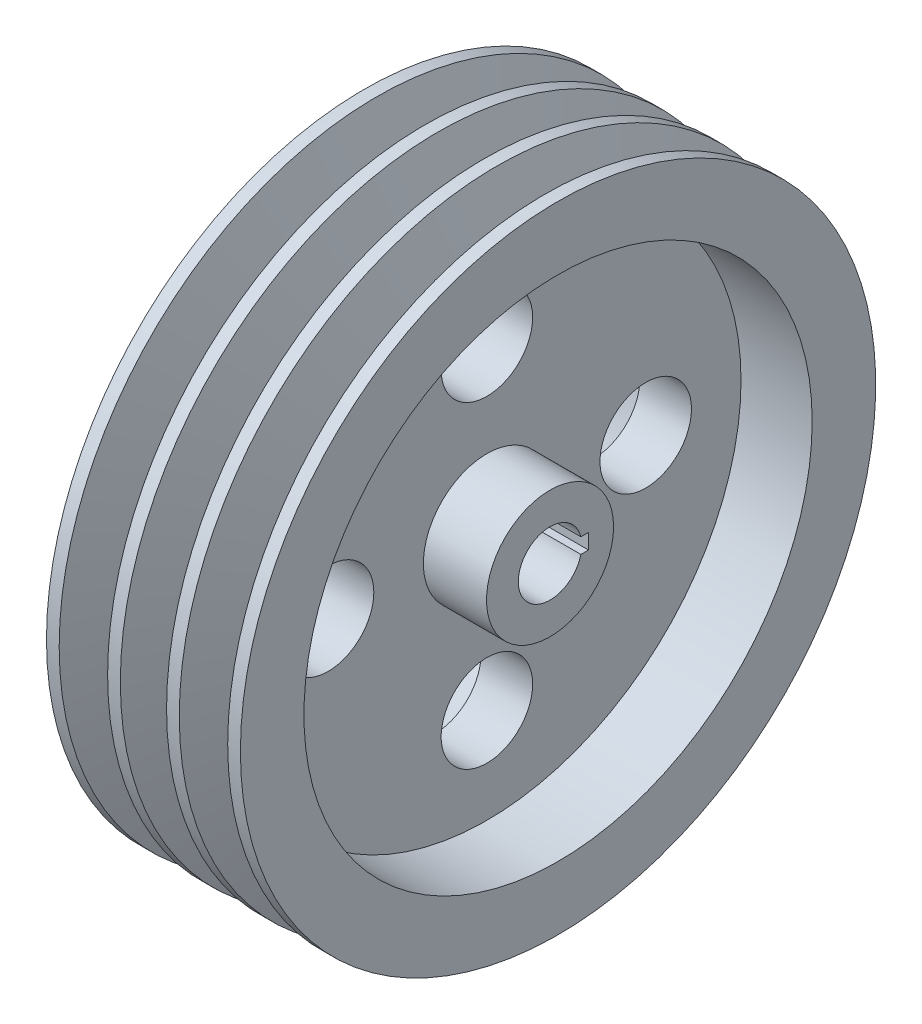
ISO-10303-21;
HEADER;
FILE_DESCRIPTION(('STEP AP214'),'2;1');
FILE_NAME('part.step','',(''),(''),'','','');
FILE_SCHEMA(('AUTOMOTIVE_DESIGN { 1 0 10303 214 1 1 1 1 }'));
ENDSEC;
DATA;
#1=APPLICATION_CONTEXT('core data for automotive mechanical design processes');
#2=APPLICATION_PROTOCOL_DEFINITION('international standard','automotive_design',2000,#1);
#3=PRODUCT_CONTEXT('',#1,'mechanical');
#4=PRODUCT('Part','Part','',(#3));
#5=PRODUCT_RELATED_PRODUCT_CATEGORY('part','',(#4));
#6=PRODUCT_DEFINITION_FORMATION('','',#4);
#7=PRODUCT_DEFINITION_CONTEXT('part definition',#1,'design');
#8=PRODUCT_DEFINITION('design','',#6,#7);
#9=PRODUCT_DEFINITION_SHAPE('','',#8);
#10=(LENGTH_UNIT() NAMED_UNIT(*) SI_UNIT(.MILLI.,.METRE.));
#11=(NAMED_UNIT(*) PLANE_ANGLE_UNIT() SI_UNIT($,.RADIAN.));
#12=(NAMED_UNIT(*) SI_UNIT($,.STERADIAN.) SOLID_ANGLE_UNIT());
#13=UNCERTAINTY_MEASURE_WITH_UNIT(LENGTH_MEASURE(1.E-05),#10,'distance_accuracy_value','');
#14=(GEOMETRIC_REPRESENTATION_CONTEXT(3) GLOBAL_UNCERTAINTY_ASSIGNED_CONTEXT((#13)) GLOBAL_UNIT_ASSIGNED_CONTEXT((#10,
#11,#12)) REPRESENTATION_CONTEXT('',''));
#15=CARTESIAN_POINT('',(0.,0.,0.));
#16=DIRECTION('',(0.,0.,1.));
#17=DIRECTION('',(1.,0.,0.));
#18=AXIS2_PLACEMENT_3D('',#15,#16,#17);
#19=CARTESIAN_POINT('',(-38.1556330512028,12.5,0.));
#20=DIRECTION('',(1.,0.,0.));
#21=DIRECTION('',(0.,0.,-1.));
#22=AXIS2_PLACEMENT_3D('',#19,#20,#21);
#23=PLANE('',#22);
#24=CARTESIAN_POINT('',(-38.1556330512028,0.,0.));
#25=DIRECTION('',(1.,0.,0.));
#26=DIRECTION('',(0.,0.,-1.));
#27=AXIS2_PLACEMENT_3D('',#24,#25,#26);
#28=CIRCLE('',#27,100.);
#29=CARTESIAN_POINT('',(-38.1556330512028,0.,-100.));
#30=VERTEX_POINT('',#29);
#31=EDGE_CURVE('E133',#30,#30,#28,.T.);
#32=ORIENTED_EDGE('',*,*,#31,.T.);
#33=EDGE_LOOP('',(#32));
#34=FACE_BOUND('',#33,.T.);
#35=CARTESIAN_POINT('',(-38.1556330512028,0.,0.));
#36=DIRECTION('',(-1.,0.,0.));
#37=DIRECTION('',(0.,0.,1.));
#38=AXIS2_PLACEMENT_3D('',#35,#36,#37);
#39=CIRCLE('',#38,125.);
#40=CARTESIAN_POINT('',(-38.1556330512028,0.,125.));
#41=VERTEX_POINT('',#40);
#42=EDGE_CURVE('E11',#41,#41,#39,.T.);
#43=ORIENTED_EDGE('',*,*,#42,.T.);
#44=EDGE_LOOP('',(#43));
#45=FACE_BOUND('',#44,.T.);
#46=ADVANCED_FACE('F39',(#34,#45),#23,.F.);
#47=CARTESIAN_POINT('',(-177.514342584117,0.,0.));
#48=DIRECTION('',(-1.,0.,0.));
#49=DIRECTION('',(0.,0.,1.));
#50=AXIS2_PLACEMENT_3D('',#47,#48,#49);
#51=CYLINDRICAL_SURFACE('',#50,125.);
#52=ORIENTED_EDGE('',*,*,#42,.F.);
#53=EDGE_LOOP('',(#52));
#54=FACE_BOUND('',#53,.T.);
#55=CARTESIAN_POINT('',(-33.1556330512028,0.,0.));
#56=DIRECTION('',(-1.,0.,0.));
#57=DIRECTION('',(0.,0.,1.));
#58=AXIS2_PLACEMENT_3D('',#55,#56,#57);
#59=CIRCLE('',#58,125.);
#60=CARTESIAN_POINT('',(-33.1556330512028,0.,125.));
#61=VERTEX_POINT('',#60);
#62=EDGE_CURVE('E50',#61,#61,#59,.T.);
#63=ORIENTED_EDGE('',*,*,#62,.T.);
#64=EDGE_LOOP('',(#63));
#65=FACE_BOUND('',#64,.T.);
#66=ADVANCED_FACE('F216',(#54,#65),#51,.T.);
#67=CARTESIAN_POINT('',(-26.6041688344111,0.,0.));
#68=DIRECTION('',(-1.,0.,0.));
#69=DIRECTION('',(0.,0.,1.));
#70=AXIS2_PLACEMENT_3D('',#67,#68,#69);
#71=CONICAL_SURFACE('',#70,107.,1.22173047639603);
#72=ORIENTED_EDGE('',*,*,#62,.F.);
#73=EDGE_LOOP('',(#72));
#74=FACE_BOUND('',#73,.T.);
#75=CARTESIAN_POINT('',(-26.6041688344111,0.,0.));
#76=DIRECTION('',(-1.,0.,0.));
#77=DIRECTION('',(0.,0.,1.));
#78=AXIS2_PLACEMENT_3D('',#75,#76,#77);
#79=CIRCLE('',#78,107.);
#80=CARTESIAN_POINT('',(-26.6041688344111,0.,107.));
#81=VERTEX_POINT('',#80);
#82=EDGE_CURVE('E177',#81,#81,#79,.T.);
#83=ORIENTED_EDGE('',*,*,#82,.T.);
#84=EDGE_LOOP('',(#83));
#85=FACE_BOUND('',#84,.T.);
#86=ADVANCED_FACE('F225',(#74,#85),#71,.T.);
#87=CARTESIAN_POINT('',(-20.629224678116,0.,0.));
#88=DIRECTION('',(1.,0.,0.));
#89=DIRECTION('',(0.,0.,-1.));
#90=AXIS2_PLACEMENT_3D('',#87,#88,#89);
#91=CONICAL_SURFACE('',#90,107.052815980487,0.00883934703360535);
#92=ORIENTED_EDGE('',*,*,#82,.F.);
#93=EDGE_LOOP('',(#92));
#94=FACE_BOUND('',#93,.T.);
#95=CARTESIAN_POINT('',(-20.629224678116,0.,0.));
#96=DIRECTION('',(-1.,0.,0.));
#97=DIRECTION('',(0.,0.,1.));
#98=AXIS2_PLACEMENT_3D('',#95,#96,#97);
#99=CIRCLE('',#98,107.052815980487);
#100=CARTESIAN_POINT('',(-20.629224678116,0.,107.052815980487));
#101=VERTEX_POINT('',#100);
#102=EDGE_CURVE('E176',#101,#101,#99,.T.);
#103=ORIENTED_EDGE('',*,*,#102,.T.);
#104=EDGE_LOOP('',(#103));
#105=FACE_BOUND('',#104,.T.);
#106=ADVANCED_FACE('F227',(#94,#105),#91,.T.);
#107=CARTESIAN_POINT('',(-14.0969839061151,0.,0.));
#108=DIRECTION('',(1.,0.,0.));
#109=DIRECTION('',(0.,0.,-1.));
#110=AXIS2_PLACEMENT_3D('',#107,#108,#109);
#111=CONICAL_SURFACE('',#110,125.,1.22173047639603);
#112=ORIENTED_EDGE('',*,*,#102,.F.);
#113=EDGE_LOOP('',(#112));
#114=FACE_BOUND('',#113,.T.);
#115=CARTESIAN_POINT('',(-14.0969839061151,0.,0.));
#116=DIRECTION('',(-1.,0.,0.));
#117=DIRECTION('',(0.,0.,1.));
#118=AXIS2_PLACEMENT_3D('',#115,#116,#117);
#119=CIRCLE('',#118,125.);
#120=CARTESIAN_POINT('',(-14.0969839061151,0.,125.));
#121=VERTEX_POINT('',#120);
#122=EDGE_CURVE('E173',#121,#121,#119,.T.);
#123=ORIENTED_EDGE('',*,*,#122,.T.);
#124=EDGE_LOOP('',(#123));
#125=FACE_BOUND('',#124,.T.);
#126=ADVANCED_FACE('F231',(#114,#125),#111,.T.);
#127=CARTESIAN_POINT('',(-177.514342584117,0.,0.));
#128=DIRECTION('',(-1.,0.,0.));
#129=DIRECTION('',(0.,0.,1.));
#130=AXIS2_PLACEMENT_3D('',#127,#128,#129);
#131=CYLINDRICAL_SURFACE('',#130,125.);
#132=ORIENTED_EDGE('',*,*,#122,.F.);
#133=EDGE_LOOP('',(#132));
#134=FACE_BOUND('',#133,.T.);
#135=CARTESIAN_POINT('',(-9.0969839061151,0.,0.));
#136=DIRECTION('',(-1.,0.,0.));
#137=DIRECTION('',(0.,0.,1.));
#138=AXIS2_PLACEMENT_3D('',#135,#136,#137);
#139=CIRCLE('',#138,125.);
#140=CARTESIAN_POINT('',(-9.0969839061151,0.,125.));
#141=VERTEX_POINT('',#140);
#142=EDGE_CURVE('E167',#141,#141,#139,.T.);
#143=ORIENTED_EDGE('',*,*,#142,.T.);
#144=EDGE_LOOP('',(#143));
#145=FACE_BOUND('',#144,.T.);
#146=ADVANCED_FACE('F237',(#134,#145),#131,.T.);
#147=CARTESIAN_POINT('',(-2.5,0.,0.));
#148=DIRECTION('',(-1.,0.,0.));
#149=DIRECTION('',(0.,0.,1.));
#150=AXIS2_PLACEMENT_3D('',#147,#148,#149);
#151=CONICAL_SURFACE('',#150,106.874935681443,1.22173047639603);
#152=ORIENTED_EDGE('',*,*,#142,.F.);
#153=EDGE_LOOP('',(#152));
#154=FACE_BOUND('',#153,.T.);
#155=CARTESIAN_POINT('',(-2.5,0.,0.));
#156=DIRECTION('',(-1.,0.,0.));
#157=DIRECTION('',(0.,0.,1.));
#158=AXIS2_PLACEMENT_3D('',#155,#156,#157);
#159=CIRCLE('',#158,106.874935681443);
#160=CARTESIAN_POINT('',(-2.5,0.,106.874935681443));
#161=VERTEX_POINT('',#160);
#162=EDGE_CURVE('E170',#161,#161,#159,.T.);
#163=ORIENTED_EDGE('',*,*,#162,.T.);
#164=EDGE_LOOP('',(#163));
#165=FACE_BOUND('',#164,.T.);
#166=ADVANCED_FACE('F244',(#154,#165),#151,.T.);
#167=CARTESIAN_POINT('',(-177.514342584117,0.,0.));
#168=DIRECTION('',(-1.,0.,0.));
#169=DIRECTION('',(0.,0.,1.));
#170=AXIS2_PLACEMENT_3D('',#167,#168,#169);
#171=CYLINDRICAL_SURFACE('',#170,106.874935681443);
#172=ORIENTED_EDGE('',*,*,#162,.F.);
#173=EDGE_LOOP('',(#172));
#174=FACE_BOUND('',#173,.T.);
#175=CARTESIAN_POINT('',(2.5,0.,0.));
#176=DIRECTION('',(-1.,0.,0.));
#177=DIRECTION('',(0.,0.,1.));
#178=AXIS2_PLACEMENT_3D('',#175,#176,#177);
#179=CIRCLE('',#178,106.874935681443);
#180=CARTESIAN_POINT('',(2.5,0.,106.874935681443));
#181=VERTEX_POINT('',#180);
#182=EDGE_CURVE('E165',#181,#181,#179,.T.);
#183=ORIENTED_EDGE('',*,*,#182,.T.);
#184=EDGE_LOOP('',(#183));
#185=FACE_BOUND('',#184,.T.);
#186=ADVANCED_FACE('F252',(#174,#185),#171,.T.);
#187=CARTESIAN_POINT('',(9.0969839061151,0.,0.));
#188=DIRECTION('',(1.,0.,0.));
#189=DIRECTION('',(0.,0.,-1.));
#190=AXIS2_PLACEMENT_3D('',#187,#188,#189);
#191=CONICAL_SURFACE('',#190,125.,1.22173047639603);
#192=ORIENTED_EDGE('',*,*,#182,.F.);
#193=EDGE_LOOP('',(#192));
#194=FACE_BOUND('',#193,.T.);
#195=CARTESIAN_POINT('',(9.0969839061151,0.,0.));
#196=DIRECTION('',(-1.,0.,0.));
#197=DIRECTION('',(0.,0.,1.));
#198=AXIS2_PLACEMENT_3D('',#195,#196,#197);
#199=CIRCLE('',#198,125.);
#200=CARTESIAN_POINT('',(9.0969839061151,0.,125.));
#201=VERTEX_POINT('',#200);
#202=EDGE_CURVE('E163',#201,#201,#199,.T.);
#203=ORIENTED_EDGE('',*,*,#202,.T.);
#204=EDGE_LOOP('',(#203));
#205=FACE_BOUND('',#204,.T.);
#206=ADVANCED_FACE('F256',(#194,#205),#191,.T.);
#207=CARTESIAN_POINT('',(-177.514342584117,0.,0.));
#208=DIRECTION('',(-1.,0.,0.));
#209=DIRECTION('',(0.,0.,1.));
#210=AXIS2_PLACEMENT_3D('',#207,#208,#209);
#211=CYLINDRICAL_SURFACE('',#210,125.);
#212=ORIENTED_EDGE('',*,*,#202,.F.);
#213=EDGE_LOOP('',(#212));
#214=FACE_BOUND('',#213,.T.);
#215=CARTESIAN_POINT('',(14.0969839061151,0.,0.));
#216=DIRECTION('',(-1.,0.,0.));
#217=DIRECTION('',(0.,0.,1.));
#218=AXIS2_PLACEMENT_3D('',#215,#216,#217);
#219=CIRCLE('',#218,125.);
#220=CARTESIAN_POINT('',(14.0969839061151,0.,125.));
#221=VERTEX_POINT('',#220);
#222=EDGE_CURVE('E156',#221,#221,#219,.T.);
#223=ORIENTED_EDGE('',*,*,#222,.T.);
#224=EDGE_LOOP('',(#223));
#225=FACE_BOUND('',#224,.T.);
#226=ADVANCED_FACE('F265',(#214,#225),#211,.T.);
#227=CARTESIAN_POINT('',(20.629224678116,0.,0.));
#228=DIRECTION('',(-1.,0.,0.));
#229=DIRECTION('',(0.,0.,1.));
#230=AXIS2_PLACEMENT_3D('',#227,#228,#229);
#231=CONICAL_SURFACE('',#230,107.052815980487,1.22173047639603);
#232=ORIENTED_EDGE('',*,*,#222,.F.);
#233=EDGE_LOOP('',(#232));
#234=FACE_BOUND('',#233,.T.);
#235=CARTESIAN_POINT('',(20.629224678116,0.,0.));
#236=DIRECTION('',(-1.,0.,0.));
#237=DIRECTION('',(0.,0.,1.));
#238=AXIS2_PLACEMENT_3D('',#235,#236,#237);
#239=CIRCLE('',#238,107.052815980487);
#240=CARTESIAN_POINT('',(20.629224678116,0.,107.052815980487));
#241=VERTEX_POINT('',#240);
#242=EDGE_CURVE('E152',#241,#241,#239,.T.);
#243=ORIENTED_EDGE('',*,*,#242,.T.);
#244=EDGE_LOOP('',(#243));
#245=FACE_BOUND('',#244,.T.);
#246=ADVANCED_FACE('F267',(#234,#245),#231,.T.);
#247=CARTESIAN_POINT('',(26.6041688344111,0.,0.));
#248=DIRECTION('',(-1.,0.,0.));
#249=DIRECTION('',(0.,0.,1.));
#250=AXIS2_PLACEMENT_3D('',#247,#248,#249);
#251=CONICAL_SURFACE('',#250,107.,0.00883934703360535);
#252=ORIENTED_EDGE('',*,*,#242,.F.);
#253=EDGE_LOOP('',(#252));
#254=FACE_BOUND('',#253,.T.);
#255=CARTESIAN_POINT('',(26.6041688344111,0.,0.));
#256=DIRECTION('',(-1.,0.,0.));
#257=DIRECTION('',(0.,0.,1.));
#258=AXIS2_PLACEMENT_3D('',#255,#256,#257);
#259=CIRCLE('',#258,107.);
#260=CARTESIAN_POINT('',(26.6041688344111,0.,107.));
#261=VERTEX_POINT('',#260);
#262=EDGE_CURVE('E151',#261,#261,#259,.T.);
#263=ORIENTED_EDGE('',*,*,#262,.T.);
#264=EDGE_LOOP('',(#263));
#265=FACE_BOUND('',#264,.T.);
#266=ADVANCED_FACE('F273',(#254,#265),#251,.T.);
#267=CARTESIAN_POINT('',(33.1556330512028,0.,0.));
#268=DIRECTION('',(1.,0.,0.));
#269=DIRECTION('',(0.,0.,-1.));
#270=AXIS2_PLACEMENT_3D('',#267,#268,#269);
#271=CONICAL_SURFACE('',#270,125.,1.22173047639603);
#272=ORIENTED_EDGE('',*,*,#262,.F.);
#273=EDGE_LOOP('',(#272));
#274=FACE_BOUND('',#273,.T.);
#275=CARTESIAN_POINT('',(33.1556330512028,0.,0.));
#276=DIRECTION('',(-1.,0.,0.));
#277=DIRECTION('',(0.,0.,1.));
#278=AXIS2_PLACEMENT_3D('',#275,#276,#277);
#279=CIRCLE('',#278,125.);
#280=CARTESIAN_POINT('',(33.1556330512028,0.,125.));
#281=VERTEX_POINT('',#280);
#282=EDGE_CURVE('E148',#281,#281,#279,.T.);
#283=ORIENTED_EDGE('',*,*,#282,.T.);
#284=EDGE_LOOP('',(#283));
#285=FACE_BOUND('',#284,.T.);
#286=ADVANCED_FACE('F284',(#274,#285),#271,.T.);
#287=CARTESIAN_POINT('',(-177.514342584117,0.,0.));
#288=DIRECTION('',(-1.,0.,0.));
#289=DIRECTION('',(0.,0.,1.));
#290=AXIS2_PLACEMENT_3D('',#287,#288,#289);
#291=CYLINDRICAL_SURFACE('',#290,125.);
#292=ORIENTED_EDGE('',*,*,#282,.F.);
#293=EDGE_LOOP('',(#292));
#294=FACE_BOUND('',#293,.T.);
#295=CARTESIAN_POINT('',(38.1556330512028,0.,0.));
#296=DIRECTION('',(-1.,0.,0.));
#297=DIRECTION('',(0.,0.,1.));
#298=AXIS2_PLACEMENT_3D('',#295,#296,#297);
#299=CIRCLE('',#298,125.);
#300=CARTESIAN_POINT('',(38.1556330512028,0.,125.));
#301=VERTEX_POINT('',#300);
#302=EDGE_CURVE('E144',#301,#301,#299,.T.);
#303=ORIENTED_EDGE('',*,*,#302,.T.);
#304=EDGE_LOOP('',(#303));
#305=FACE_BOUND('',#304,.T.);
#306=ADVANCED_FACE('F290',(#294,#305),#291,.T.);
#307=CARTESIAN_POINT('',(38.1556330512028,12.5,0.));
#308=DIRECTION('',(-1.,0.,0.));
#309=DIRECTION('',(0.,0.,1.));
#310=AXIS2_PLACEMENT_3D('',#307,#308,#309);
#311=PLANE('',#310);
#312=CARTESIAN_POINT('',(38.1556330512028,0.,0.));
#313=DIRECTION('',(1.,0.,0.));
#314=DIRECTION('',(0.,0.,-1.));
#315=AXIS2_PLACEMENT_3D('',#312,#313,#314);
#316=CIRCLE('',#315,100.);
#317=CARTESIAN_POINT('',(38.1556330512028,0.,-100.));
#318=VERTEX_POINT('',#317);
#319=EDGE_CURVE('E136',#318,#318,#316,.T.);
#320=ORIENTED_EDGE('',*,*,#319,.F.);
#321=EDGE_LOOP('',(#320));
#322=FACE_BOUND('',#321,.T.);
#323=ORIENTED_EDGE('',*,*,#302,.F.);
#324=EDGE_LOOP('',(#323));
#325=FACE_BOUND('',#324,.T.);
#326=ADVANCED_FACE('F291',(#322,#325),#311,.F.);
#327=CARTESIAN_POINT('',(10.1556330512028,0.,0.));
#328=DIRECTION('',(1.,0.,0.));
#329=DIRECTION('',(0.,0.,-1.));
#330=AXIS2_PLACEMENT_3D('',#327,#328,#329);
#331=PLANE('',#330);
#332=CARTESIAN_POINT('',(10.1556330512028,0.,0.));
#333=DIRECTION('',(1.,0.,0.));
#334=DIRECTION('',(0.,0.,-1.));
#335=AXIS2_PLACEMENT_3D('',#332,#333,#334);
#336=CIRCLE('',#335,25.);
#337=CARTESIAN_POINT('',(10.1556330512028,0.,-25.));
#338=VERTEX_POINT('',#337);
#339=EDGE_CURVE('E114',#338,#338,#336,.F.);
#340=ORIENTED_EDGE('',*,*,#339,.T.);
#341=EDGE_LOOP('',(#340));
#342=FACE_BOUND('',#341,.T.);
#343=CARTESIAN_POINT('',(10.1556330512028,62.5,0.));
#344=DIRECTION('',(1.,0.,0.));
#345=DIRECTION('',(0.,0.,-1.));
#346=AXIS2_PLACEMENT_3D('',#343,#344,#345);
#347=CIRCLE('',#346,18.);
#348=CARTESIAN_POINT('',(10.1556330512028,62.5,-18.));
#349=VERTEX_POINT('',#348);
#350=EDGE_CURVE('E134',#349,#349,#347,.T.);
#351=ORIENTED_EDGE('',*,*,#350,.F.);
#352=EDGE_LOOP('',(#351));
#353=FACE_BOUND('',#352,.T.);
#354=CARTESIAN_POINT('',(10.1556330512028,3.5412326150585E-12,-62.5000000000035));
#355=DIRECTION('',(1.,0.,0.));
#356=DIRECTION('',(0.,0.,-1.));
#357=AXIS2_PLACEMENT_3D('',#354,#355,#356);
#358=CIRCLE('',#357,18.0000000000026);
#359=CARTESIAN_POINT('',(10.1556330512028,3.5412326150585E-12,-80.5000000000061));
#360=VERTEX_POINT('',#359);
#361=EDGE_CURVE('E126',#360,#360,#358,.T.);
#362=ORIENTED_EDGE('',*,*,#361,.F.);
#363=EDGE_LOOP('',(#362));
#364=FACE_BOUND('',#363,.T.);
#365=CARTESIAN_POINT('',(10.1556330512028,-62.5,-7.08246523011699E-12));
#366=DIRECTION('',(1.,0.,0.));
#367=DIRECTION('',(0.,0.,-1.));
#368=AXIS2_PLACEMENT_3D('',#365,#366,#367);
#369=CIRCLE('',#368,18.0000000000072);
#370=CARTESIAN_POINT('',(10.1556330512028,-62.5,-18.0000000000143));
#371=VERTEX_POINT('',#370);
#372=EDGE_CURVE('E124',#371,#371,#369,.T.);
#373=ORIENTED_EDGE('',*,*,#372,.F.);
#374=EDGE_LOOP('',(#373));
#375=FACE_BOUND('',#374,.T.);
#376=CARTESIAN_POINT('',(10.1556330512028,-3.54888665755317E-12,62.4999999999965));
#377=DIRECTION('',(1.,0.,0.));
#378=DIRECTION('',(0.,0.,-1.));
#379=AXIS2_PLACEMENT_3D('',#376,#377,#378);
#380=CIRCLE('',#379,18.0000000000051);
#381=CARTESIAN_POINT('',(10.1556330512028,-3.54888665755317E-12,44.4999999999914));
#382=VERTEX_POINT('',#381);
#383=EDGE_CURVE('E118',#382,#382,#380,.T.);
#384=ORIENTED_EDGE('',*,*,#383,.F.);
#385=EDGE_LOOP('',(#384));
#386=FACE_BOUND('',#385,.T.);
#387=CARTESIAN_POINT('',(10.1556330512028,0.,0.));
#388=DIRECTION('',(1.,0.,0.));
#389=DIRECTION('',(0.,0.,-1.));
#390=AXIS2_PLACEMENT_3D('',#387,#388,#389);
#391=CIRCLE('',#390,100.);
#392=CARTESIAN_POINT('',(10.1556330512028,0.,-100.));
#393=VERTEX_POINT('',#392);
#394=EDGE_CURVE('E142',#393,#393,#391,.T.);
#395=ORIENTED_EDGE('',*,*,#394,.T.);
#396=EDGE_LOOP('',(#395));
#397=FACE_BOUND('',#396,.T.);
#398=ADVANCED_FACE('F296',(#342,#353,#364,#375,#386,#397),#331,.T.);
#399=CARTESIAN_POINT('',(10.1556330512028,0.,0.));
#400=DIRECTION('',(1.,0.,0.));
#401=DIRECTION('',(0.,0.,-1.));
#402=AXIS2_PLACEMENT_3D('',#399,#400,#401);
#403=CYLINDRICAL_SURFACE('',#402,100.);
#404=ORIENTED_EDGE('',*,*,#394,.F.);
#405=EDGE_LOOP('',(#404));
#406=FACE_BOUND('',#405,.T.);
#407=ORIENTED_EDGE('',*,*,#319,.T.);
#408=EDGE_LOOP('',(#407));
#409=FACE_BOUND('',#408,.T.);
#410=ADVANCED_FACE('F200',(#406,#409),#403,.F.);
#411=CARTESIAN_POINT('',(-10.1556330512028,0.,0.));
#412=DIRECTION('',(-1.,0.,0.));
#413=DIRECTION('',(0.,0.,-1.));
#414=AXIS2_PLACEMENT_3D('',#411,#412,#413);
#415=PLANE('',#414);
#416=CARTESIAN_POINT('',(-10.1556330512028,0.,0.));
#417=DIRECTION('',(-1.,0.,0.));
#418=DIRECTION('',(0.,0.,1.));
#419=AXIS2_PLACEMENT_3D('',#416,#417,#418);
#420=CIRCLE('',#419,25.);
#421=CARTESIAN_POINT('',(-10.1556330512028,0.,25.));
#422=VERTEX_POINT('',#421);
#423=EDGE_CURVE('E45',#422,#422,#420,.F.);
#424=ORIENTED_EDGE('',*,*,#423,.T.);
#425=EDGE_LOOP('',(#424));
#426=FACE_BOUND('',#425,.T.);
#427=CARTESIAN_POINT('',(-10.1556330512028,62.5,0.));
#428=DIRECTION('',(-1.,0.,0.));
#429=DIRECTION('',(0.,0.,1.));
#430=AXIS2_PLACEMENT_3D('',#427,#428,#429);
#431=CIRCLE('',#430,18.);
#432=CARTESIAN_POINT('',(-10.1556330512028,62.5,18.));
#433=VERTEX_POINT('',#432);
#434=EDGE_CURVE('E127',#433,#433,#431,.T.);
#435=ORIENTED_EDGE('',*,*,#434,.F.);
#436=EDGE_LOOP('',(#435));
#437=FACE_BOUND('',#436,.T.);
#438=CARTESIAN_POINT('',(-10.1556330512028,3.5412326150585E-12,-62.5000000000035));
#439=DIRECTION('',(-1.,0.,0.));
#440=DIRECTION('',(0.,0.,1.));
#441=AXIS2_PLACEMENT_3D('',#438,#439,#440);
#442=CIRCLE('',#441,18.0000000000026);
#443=CARTESIAN_POINT('',(-10.1556330512028,3.5412326150585E-12,-44.500000000001));
#444=VERTEX_POINT('',#443);
#445=EDGE_CURVE('E129',#444,#444,#442,.T.);
#446=ORIENTED_EDGE('',*,*,#445,.F.);
#447=EDGE_LOOP('',(#446));
#448=FACE_BOUND('',#447,.T.);
#449=CARTESIAN_POINT('',(-10.1556330512028,-62.5,-7.08246523011699E-12));
#450=DIRECTION('',(-1.,0.,0.));
#451=DIRECTION('',(0.,0.,1.));
#452=AXIS2_PLACEMENT_3D('',#449,#450,#451);
#453=CIRCLE('',#452,18.0000000000072);
#454=CARTESIAN_POINT('',(-10.1556330512028,-62.5,18.0000000000001));
#455=VERTEX_POINT('',#454);
#456=EDGE_CURVE('E125',#455,#455,#453,.T.);
#457=ORIENTED_EDGE('',*,*,#456,.F.);
#458=EDGE_LOOP('',(#457));
#459=FACE_BOUND('',#458,.T.);
#460=CARTESIAN_POINT('',(-10.1556330512028,-3.54888665755317E-12,62.4999999999965));
#461=DIRECTION('',(-1.,0.,0.));
#462=DIRECTION('',(0.,0.,1.));
#463=AXIS2_PLACEMENT_3D('',#460,#461,#462);
#464=CIRCLE('',#463,18.0000000000051);
#465=CARTESIAN_POINT('',(-10.1556330512028,-3.54888665755317E-12,80.5000000000015));
#466=VERTEX_POINT('',#465);
#467=EDGE_CURVE('E117',#466,#466,#464,.T.);
#468=ORIENTED_EDGE('',*,*,#467,.F.);
#469=EDGE_LOOP('',(#468));
#470=FACE_BOUND('',#469,.T.);
#471=CARTESIAN_POINT('',(-10.1556330512028,0.,0.));
#472=DIRECTION('',(1.,0.,0.));
#473=DIRECTION('',(0.,0.,-1.));
#474=AXIS2_PLACEMENT_3D('',#471,#472,#473);
#475=CIRCLE('',#474,100.);
#476=CARTESIAN_POINT('',(-10.1556330512028,0.,-100.));
#477=VERTEX_POINT('',#476);
#478=EDGE_CURVE('E132',#477,#477,#475,.T.);
#479=ORIENTED_EDGE('',*,*,#478,.F.);
#480=EDGE_LOOP('',(#479));
#481=FACE_BOUND('',#480,.T.);
#482=ADVANCED_FACE('F193',(#426,#437,#448,#459,#470,#481),#415,.T.);
#483=CARTESIAN_POINT('',(-10.1556330512028,0.,0.));
#484=DIRECTION('',(-1.,0.,0.));
#485=DIRECTION('',(0.,0.,1.));
#486=AXIS2_PLACEMENT_3D('',#483,#484,#485);
#487=CYLINDRICAL_SURFACE('',#486,100.);
#488=ORIENTED_EDGE('',*,*,#478,.T.);
#489=EDGE_LOOP('',(#488));
#490=FACE_BOUND('',#489,.T.);
#491=ORIENTED_EDGE('',*,*,#31,.F.);
#492=EDGE_LOOP('',(#491));
#493=FACE_BOUND('',#492,.T.);
#494=ADVANCED_FACE('F196',(#490,#493),#487,.F.);
#495=CARTESIAN_POINT('',(-11.,-3.54888665755317E-12,62.4999999999965));
#496=DIRECTION('',(1.,0.,0.));
#497=DIRECTION('',(0.,0.,-1.));
#498=AXIS2_PLACEMENT_3D('',#495,#496,#497);
#499=CYLINDRICAL_SURFACE('',#498,18.0000000000051);
#500=ORIENTED_EDGE('',*,*,#383,.T.);
#501=EDGE_LOOP('',(#500));
#502=FACE_BOUND('',#501,.T.);
#503=ORIENTED_EDGE('',*,*,#467,.T.);
#504=EDGE_LOOP('',(#503));
#505=FACE_BOUND('',#504,.T.);
#506=ADVANCED_FACE('F214',(#502,#505),#499,.F.);
#507=CARTESIAN_POINT('',(-11.,-62.5,-7.08246523011699E-12));
#508=DIRECTION('',(1.,0.,0.));
#509=DIRECTION('',(0.,0.,-1.));
#510=AXIS2_PLACEMENT_3D('',#507,#508,#509);
#511=CYLINDRICAL_SURFACE('',#510,18.0000000000072);
#512=ORIENTED_EDGE('',*,*,#372,.T.);
#513=EDGE_LOOP('',(#512));
#514=FACE_BOUND('',#513,.T.);
#515=ORIENTED_EDGE('',*,*,#456,.T.);
#516=EDGE_LOOP('',(#515));
#517=FACE_BOUND('',#516,.T.);
#518=ADVANCED_FACE('F312',(#514,#517),#511,.F.);
#519=CARTESIAN_POINT('',(-11.,3.5412326150585E-12,-62.5000000000035));
#520=DIRECTION('',(1.,0.,0.));
#521=DIRECTION('',(0.,0.,-1.));
#522=AXIS2_PLACEMENT_3D('',#519,#520,#521);
#523=CYLINDRICAL_SURFACE('',#522,18.0000000000026);
#524=ORIENTED_EDGE('',*,*,#361,.T.);
#525=EDGE_LOOP('',(#524));
#526=FACE_BOUND('',#525,.T.);
#527=ORIENTED_EDGE('',*,*,#445,.T.);
#528=EDGE_LOOP('',(#527));
#529=FACE_BOUND('',#528,.T.);
#530=ADVANCED_FACE('F320',(#526,#529),#523,.F.);
#531=CARTESIAN_POINT('',(-11.,62.5,0.));
#532=DIRECTION('',(1.,0.,0.));
#533=DIRECTION('',(0.,0.,-1.));
#534=AXIS2_PLACEMENT_3D('',#531,#532,#533);
#535=CYLINDRICAL_SURFACE('',#534,18.);
#536=ORIENTED_EDGE('',*,*,#350,.T.);
#537=EDGE_LOOP('',(#536));
#538=FACE_BOUND('',#537,.T.);
#539=ORIENTED_EDGE('',*,*,#434,.T.);
#540=EDGE_LOOP('',(#539));
#541=FACE_BOUND('',#540,.T.);
#542=ADVANCED_FACE('F191',(#538,#541),#535,.F.);
#543=CARTESIAN_POINT('',(-35.,0.,0.));
#544=DIRECTION('',(1.,0.,0.));
#545=DIRECTION('',(0.,0.,-1.));
#546=AXIS2_PLACEMENT_3D('',#543,#544,#545);
#547=PLANE('',#546);
#548=CARTESIAN_POINT('',(-35.,0.,0.));
#549=DIRECTION('',(1.,0.,0.));
#550=DIRECTION('',(0.,0.,-1.));
#551=AXIS2_PLACEMENT_3D('',#548,#549,#550);
#552=CIRCLE('',#551,12.5);
#553=CARTESIAN_POINT('',(-35.,3.,-12.1346610995116));
#554=VERTEX_POINT('',#553);
#555=CARTESIAN_POINT('',(-35.,-3.,-12.1346610995116));
#556=VERTEX_POINT('',#555);
#557=EDGE_CURVE('E96',#554,#556,#552,.T.);
#558=ORIENTED_EDGE('',*,*,#557,.T.);
#559=DIRECTION('',(0.,0.,-1.));
#560=VECTOR('',#559,1.);
#561=CARTESIAN_POINT('',(-35.,-3.,-15.1346610995116));
#562=LINE('',#561,#560);
#563=CARTESIAN_POINT('',(-35.,-3.,-15.1346610995116));
#564=VERTEX_POINT('',#563);
#565=EDGE_CURVE('E99',#556,#564,#562,.T.);
#566=ORIENTED_EDGE('',*,*,#565,.T.);
#567=DIRECTION('',(0.,1.,0.));
#568=VECTOR('',#567,1.);
#569=CARTESIAN_POINT('',(-35.,3.,-15.1346610995116));
#570=LINE('',#569,#568);
#571=CARTESIAN_POINT('',(-35.,3.,-15.1346610995116));
#572=VERTEX_POINT('',#571);
#573=EDGE_CURVE('E100',#564,#572,#570,.T.);
#574=ORIENTED_EDGE('',*,*,#573,.T.);
#575=DIRECTION('',(0.,0.,1.));
#576=VECTOR('',#575,1.);
#577=CARTESIAN_POINT('',(-35.,3.,-15.1346610995116));
#578=LINE('',#577,#576);
#579=EDGE_CURVE('E82',#572,#554,#578,.T.);
#580=ORIENTED_EDGE('',*,*,#579,.T.);
#581=EDGE_LOOP('',(#558,#566,#574,#580));
#582=FACE_BOUND('',#581,.T.);
#583=CARTESIAN_POINT('',(-35.,0.,0.));
#584=DIRECTION('',(1.,0.,0.));
#585=DIRECTION('',(0.,0.,-1.));
#586=AXIS2_PLACEMENT_3D('',#583,#584,#585);
#587=CIRCLE('',#586,25.);
#588=CARTESIAN_POINT('',(-35.,0.,-25.));
#589=VERTEX_POINT('',#588);
#590=EDGE_CURVE('E104',#589,#589,#587,.T.);
#591=ORIENTED_EDGE('',*,*,#590,.F.);
#592=EDGE_LOOP('',(#591));
#593=FACE_BOUND('',#592,.T.);
#594=ADVANCED_FACE('F94',(#582,#593),#547,.F.);
#595=CARTESIAN_POINT('',(35.,0.,0.));
#596=DIRECTION('',(-1.,0.,0.));
#597=DIRECTION('',(0.,0.,1.));
#598=AXIS2_PLACEMENT_3D('',#595,#596,#597);
#599=CYLINDRICAL_SURFACE('',#598,25.);
#600=ORIENTED_EDGE('',*,*,#423,.F.);
#601=EDGE_LOOP('',(#600));
#602=FACE_BOUND('',#601,.T.);
#603=ORIENTED_EDGE('',*,*,#590,.T.);
#604=EDGE_LOOP('',(#603));
#605=FACE_BOUND('',#604,.T.);
#606=ADVANCED_FACE('F322',(#602,#605),#599,.T.);
#607=ORIENTED_EDGE('',*,*,#339,.F.);
#608=EDGE_LOOP('',(#607));
#609=FACE_BOUND('',#608,.T.);
#610=CARTESIAN_POINT('',(35.,0.,0.));
#611=DIRECTION('',(1.,0.,0.));
#612=DIRECTION('',(0.,0.,-1.));
#613=AXIS2_PLACEMENT_3D('',#610,#611,#612);
#614=CIRCLE('',#613,25.);
#615=CARTESIAN_POINT('',(35.,0.,-25.));
#616=VERTEX_POINT('',#615);
#617=EDGE_CURVE('E108',#616,#616,#614,.T.);
#618=ORIENTED_EDGE('',*,*,#617,.F.);
#619=EDGE_LOOP('',(#618));
#620=FACE_BOUND('',#619,.T.);
#621=ADVANCED_FACE('F330',(#609,#620),#599,.T.);
#622=CARTESIAN_POINT('',(35.,0.,0.));
#623=DIRECTION('',(1.,0.,0.));
#624=DIRECTION('',(0.,0.,-1.));
#625=AXIS2_PLACEMENT_3D('',#622,#623,#624);
#626=PLANE('',#625);
#627=DIRECTION('',(0.,0.,-1.));
#628=VECTOR('',#627,1.);
#629=CARTESIAN_POINT('',(35.,-3.,-15.1346610995116));
#630=LINE('',#629,#628);
#631=CARTESIAN_POINT('',(35.,-3.,-12.1346610995116));
#632=VERTEX_POINT('',#631);
#633=CARTESIAN_POINT('',(35.,-3.,-15.1346610995116));
#634=VERTEX_POINT('',#633);
#635=EDGE_CURVE('E350',#632,#634,#630,.T.);
#636=ORIENTED_EDGE('',*,*,#635,.F.);
#637=CARTESIAN_POINT('',(35.,0.,0.));
#638=DIRECTION('',(1.,0.,0.));
#639=DIRECTION('',(0.,0.,-1.));
#640=AXIS2_PLACEMENT_3D('',#637,#638,#639);
#641=CIRCLE('',#640,12.5);
#642=CARTESIAN_POINT('',(35.,3.,-12.1346610995116));
#643=VERTEX_POINT('',#642);
#644=EDGE_CURVE('E102',#643,#632,#641,.T.);
#645=ORIENTED_EDGE('',*,*,#644,.F.);
#646=DIRECTION('',(0.,0.,1.));
#647=VECTOR('',#646,1.);
#648=CARTESIAN_POINT('',(35.,3.,-15.1346610995116));
#649=LINE('',#648,#647);
#650=CARTESIAN_POINT('',(35.,3.,-15.1346610995116));
#651=VERTEX_POINT('',#650);
#652=EDGE_CURVE('E54',#651,#643,#649,.T.);
#653=ORIENTED_EDGE('',*,*,#652,.F.);
#654=DIRECTION('',(0.,1.,0.));
#655=VECTOR('',#654,1.);
#656=CARTESIAN_POINT('',(35.,3.,-15.1346610995116));
#657=LINE('',#656,#655);
#658=EDGE_CURVE('E353',#634,#651,#657,.T.);
#659=ORIENTED_EDGE('',*,*,#658,.F.);
#660=EDGE_LOOP('',(#636,#645,#653,#659));
#661=FACE_BOUND('',#660,.T.);
#662=ORIENTED_EDGE('',*,*,#617,.T.);
#663=EDGE_LOOP('',(#662));
#664=FACE_BOUND('',#663,.T.);
#665=ADVANCED_FACE('F335',(#661,#664),#626,.T.);
#666=CARTESIAN_POINT('',(-35.,0.,0.));
#667=DIRECTION('',(1.,0.,0.));
#668=DIRECTION('',(0.,0.,-1.));
#669=AXIS2_PLACEMENT_3D('',#666,#667,#668);
#670=CYLINDRICAL_SURFACE('',#669,12.5);
#671=ORIENTED_EDGE('',*,*,#644,.T.);
#672=DIRECTION('',(1.,0.,0.));
#673=VECTOR('',#672,1.);
#674=CARTESIAN_POINT('',(-35.,-3.,-12.1346610995116));
#675=LINE('',#674,#673);
#676=EDGE_CURVE('E93',#556,#632,#675,.T.);
#677=ORIENTED_EDGE('',*,*,#676,.F.);
#678=ORIENTED_EDGE('',*,*,#557,.F.);
#679=DIRECTION('',(1.,0.,0.));
#680=VECTOR('',#679,1.);
#681=CARTESIAN_POINT('',(-35.,3.,-12.1346610995116));
#682=LINE('',#681,#680);
#683=EDGE_CURVE('E81',#554,#643,#682,.T.);
#684=ORIENTED_EDGE('',*,*,#683,.T.);
#685=EDGE_LOOP('',(#671,#677,#678,#684));
#686=FACE_BOUND('',#685,.T.);
#687=ADVANCED_FACE('F101',(#686),#670,.F.);
#688=CARTESIAN_POINT('',(-35.,3.,-15.1346610995116));
#689=DIRECTION('',(0.,0.,-1.));
#690=DIRECTION('',(-1.,0.,0.));
#691=AXIS2_PLACEMENT_3D('',#688,#689,#690);
#692=PLANE('',#691);
#693=ORIENTED_EDGE('',*,*,#658,.T.);
#694=DIRECTION('',(1.,0.,0.));
#695=VECTOR('',#694,1.);
#696=CARTESIAN_POINT('',(-35.,3.,-15.1346610995116));
#697=LINE('',#696,#695);
#698=EDGE_CURVE('E78',#572,#651,#697,.T.);
#699=ORIENTED_EDGE('',*,*,#698,.F.);
#700=ORIENTED_EDGE('',*,*,#573,.F.);
#701=DIRECTION('',(1.,0.,0.));
#702=VECTOR('',#701,1.);
#703=CARTESIAN_POINT('',(-35.,-3.,-15.1346610995116));
#704=LINE('',#703,#702);
#705=EDGE_CURVE('E63',#564,#634,#704,.T.);
#706=ORIENTED_EDGE('',*,*,#705,.T.);
#707=EDGE_LOOP('',(#693,#699,#700,#706));
#708=FACE_BOUND('',#707,.T.);
#709=ADVANCED_FACE('F336',(#708),#692,.F.);
#710=CARTESIAN_POINT('',(-35.,-3.,-15.1346610995116));
#711=DIRECTION('',(0.,-1.,0.));
#712=DIRECTION('',(0.,0.,-1.));
#713=AXIS2_PLACEMENT_3D('',#710,#711,#712);
#714=PLANE('',#713);
#715=ORIENTED_EDGE('',*,*,#635,.T.);
#716=ORIENTED_EDGE('',*,*,#705,.F.);
#717=ORIENTED_EDGE('',*,*,#565,.F.);
#718=ORIENTED_EDGE('',*,*,#676,.T.);
#719=EDGE_LOOP('',(#715,#716,#717,#718));
#720=FACE_BOUND('',#719,.T.);
#721=ADVANCED_FACE('F344',(#720),#714,.F.);
#722=CARTESIAN_POINT('',(-35.,3.,-15.1346610995116));
#723=DIRECTION('',(0.,1.,0.));
#724=DIRECTION('',(0.,0.,1.));
#725=AXIS2_PLACEMENT_3D('',#722,#723,#724);
#726=PLANE('',#725);
#727=ORIENTED_EDGE('',*,*,#652,.T.);
#728=ORIENTED_EDGE('',*,*,#683,.F.);
#729=ORIENTED_EDGE('',*,*,#579,.F.);
#730=ORIENTED_EDGE('',*,*,#698,.T.);
#731=EDGE_LOOP('',(#727,#728,#729,#730));
#732=FACE_BOUND('',#731,.T.);
#733=ADVANCED_FACE('F83',(#732),#726,.F.);
#734=CLOSED_SHELL('',(#46,#66,#86,#106,#126,#146,#166,#186,#206,#226,#246,#266,#286,#306,#326,
#398,#410,#482,#494,#506,#518,#530,#542,#594,#606,#621,#665,#687,#709,#721,#733));
#735=MANIFOLD_SOLID_BREP('B2',#734);
#736=ADVANCED_BREP_SHAPE_REPRESENTATION('',(#18,#735),#14);
#737=SHAPE_DEFINITION_REPRESENTATION(#9,#736);
ENDSEC;
END-ISO-10303-21;
